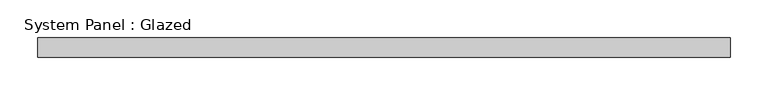
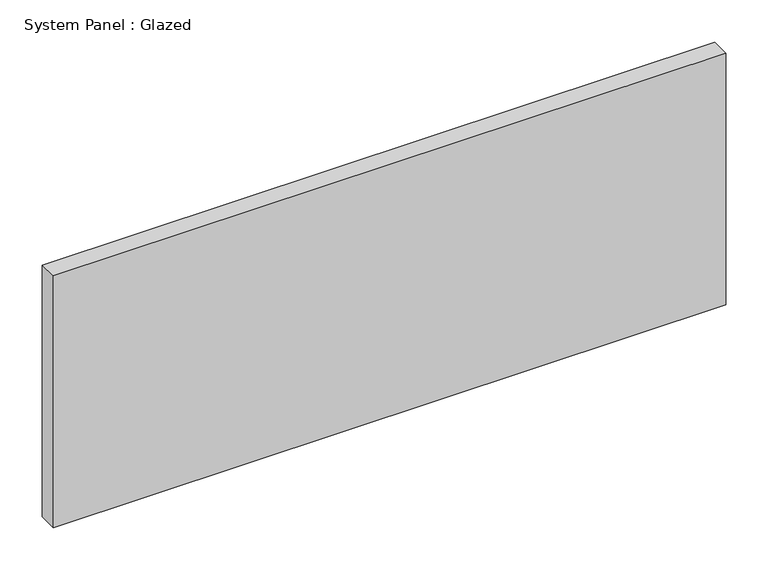
"""IFC4 building model written with IfcOpenShell, lengths in millimetres: plate geometry, System Panel : Glazed."""

from ifc_helpers import new_model, si_unit, origin, origin_with_axes, place, context, project, spatial, polyline, outline, extrude, source, transform, mapped, element, save


def system_panel_glazed_bdb1f896(model_context):
    return source(origin(), model_context, "Body", "SweptSolid", [
        extrude(outline(polyline([(457.2, 19.05), (-457.2, 19.05), (-457.2, 44.45), (457.2, 44.45), (457.2, 19.05)])), origin_with_axes(), (0.0, 0.0, 1.0), 361.95),
    ])


if __name__ == "__main__":
    model = new_model("IFC4")
    model_context = context("Model", 3, world=origin())
    ifc_project = project(units=[si_unit("LENGTHUNIT", "METRE", prefix="MILLI")], contexts=[model_context])
    site = spatial("IfcSite", under=ifc_project)
    building = spatial("IfcBuilding", under=site)
    placement = place(None, origin())
    system_panel_glazed_shape = system_panel_glazed_bdb1f896(model_context)
    element("IfcPlate", 1, ObjectType="System Panel : Glazed", at=placement, inside=building, context=model_context, shape_type="MappedRepresentation", body=[
        mapped(system_panel_glazed_shape, transform((0.0, 0.0, 0.0), x_axis=(1.0, 0.0, 0.0), y_axis=(0.0, 1.0, 0.0), z_axis=(0.0, 0.0, 1.0))),
    ])
    save(model, "model.ifc")

# Revit data of these elements
# Type "System Panel : Glazed"
#   Construction Type Id = "GSP4R"
#   Analytic Construction = "1/8 in Pilkington single glazing"
#   Visual Light Transmittance = 0.9
#   Solar Heat Gain Coefficient = 0.86
#   Heat Transfer Coefficient (U) = 1.18115 BTU/(h·ft²·°F)
# Element 1 (IfcPlate, "System Panel : Glazed")
#   Materials on its faces: "Glass"
# Materials
#   "Glass": class "Glass", colour RGB 0 128 192, transparency 0.75, Description = "Soda Lime Glass", Cost = 0
